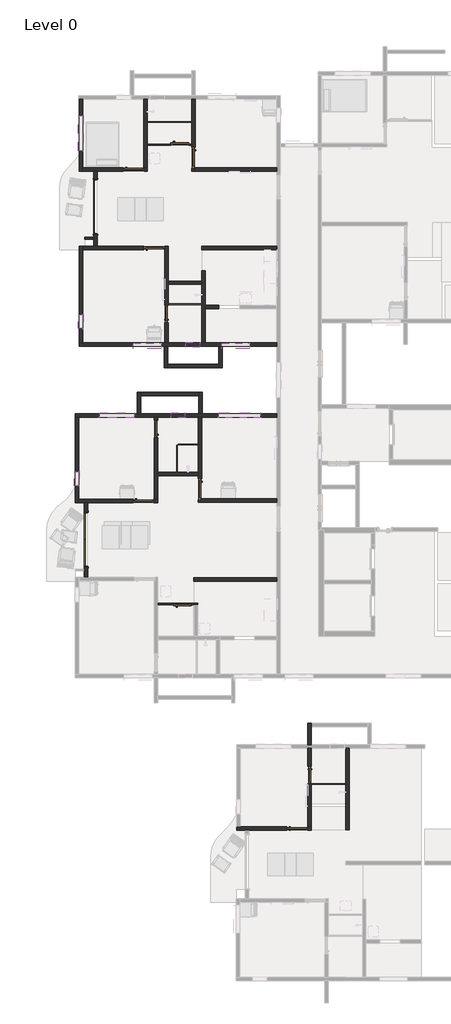
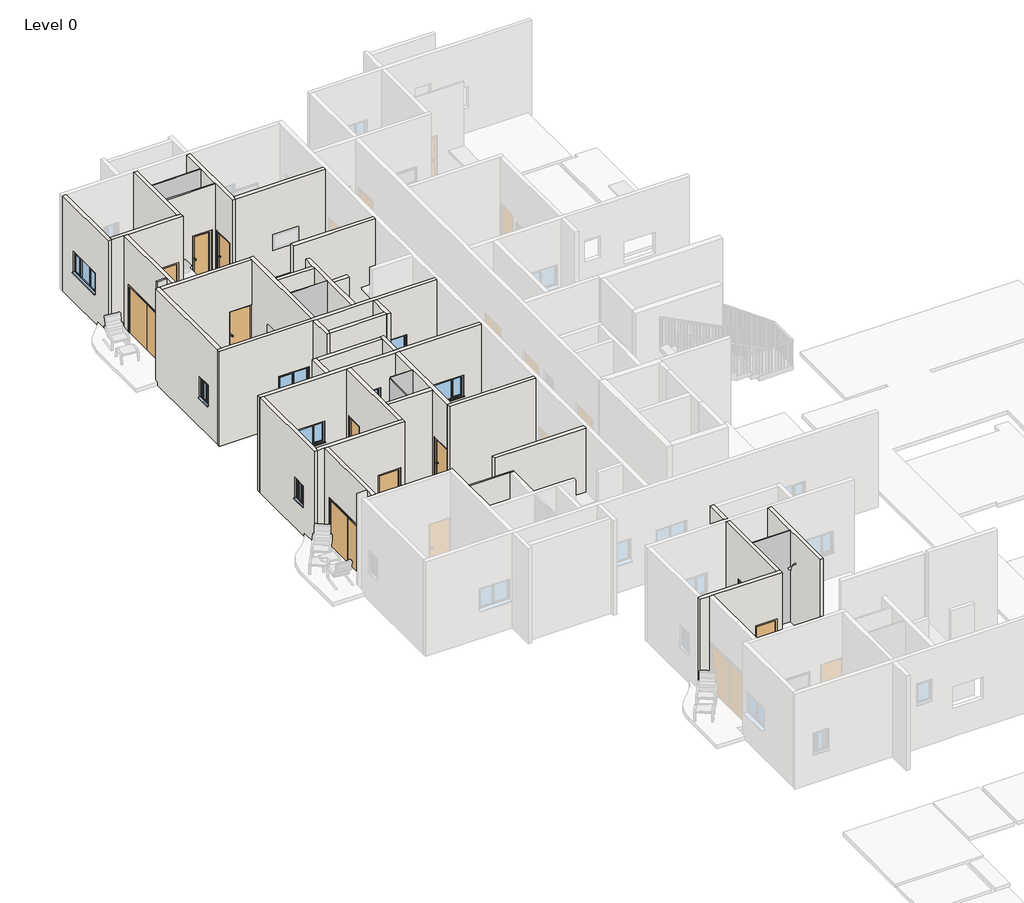
# One storey, part 4 of 14: 35 walls, 14 doors, 9 windows, 5 plates.
"""IFC4 building model written with IfcOpenShell, lengths in millimetres."""

from ifc_helpers import new_model, si_unit, frame, origin, origin_with_axes, place, context, project, spatial, polyline, outline, extrude, faceted_brep, transform, mapped, element, save
from components import doors_concept_intdbl_8_5090a96f, doors_extsgl_flush_d2_fac1298c, doors_extsgl_flush_d2_5e0ff3e2, doors_extsgl_flush_d3_352cde1d, doors_extsgl_flush_d3_ba5ff989, doors_extsgl_flush_d3_fcdd24de, doors_extsgl_flush_d3_225e8ac6, system_panel_glazed_095a6893, system_panel_glazed_930ddd10, system_panel_glazed_c2994357, system_panel_glazed_5123bacf, system_panel_glazed_5cf703a3, windows_concept_plain_dbl_4_d1e2e333, windows_sgl_plain_2_be143095, windows_tpl_variable_casement_2_47b04551, windows_tpl_variable_casement_5_ffad3fa3, windows_tpl_variable_casement_6_d811e495

model = new_model("IFC4")

# Units and contexts
model_context = context("Model", 3, world=origin())
ifc_project = project(units=[si_unit("LENGTHUNIT", "METRE", prefix="MILLI")], contexts=[model_context])

# Site, building, storey
site = spatial("IfcSite", under=ifc_project)
building = spatial("IfcBuilding", under=site)
storey = spatial("IfcBuildingStorey", under=building, Name="Level 0", Elevation=0.0)

# Doors
placement = place(None, origin())
doors_concept_intdbl_8_shape = doors_concept_intdbl_8_5090a96f(model_context)
element("IfcDoor", 1, ObjectType="Doors_Concept_IntDbl : 8'", at=placement, inside=storey, context=model_context, shape_type="MappedRepresentation", body=[
    mapped(doors_concept_intdbl_8_shape, transform((-38935.3458282, 59742.2966928, 0.0), x_axis=(0.0, 1.0, 0.0), y_axis=(-1.0, 0.0, 0.0), z_axis=(0.0, 0.0, 1.0))),
])
element("IfcDoor", 2, ObjectType="Doors_Concept_IntDbl : 8'", at=placement, inside=storey, context=model_context, shape_type="MappedRepresentation", body=[
    mapped(doors_concept_intdbl_8_shape, transform((-39340.8800447, 45143.1998557, 0.0), x_axis=(0.0, 1.0, 0.0), y_axis=(-1.0, 0.0, 0.0), z_axis=(0.0, 0.0, 1.0))),
])
doors_extsgl_flush_d2_shape = doors_extsgl_flush_d2_fac1298c(model_context)
element("IfcDoor", 3, ObjectType="Doors_ExtSgl_Flush : D2", at=placement, inside=storey, context=model_context, shape_type="MappedRepresentation", body=[
    mapped(doors_extsgl_flush_d2_shape, transform((-30080.8505269, 32458.2541094, 0.0), x_axis=(1.0, 0.0, 0.0), y_axis=(0.0, 1.0, 0.0), z_axis=(0.0, 0.0, 1.0))),
])
element("IfcDoor", 4, ObjectType="Doors_ExtSgl_Flush : D2", at=placement, inside=storey, context=model_context, shape_type="MappedRepresentation", body=[
    mapped(doors_extsgl_flush_d2_shape, transform((-36827.1458282, 46838.6498557, 0.0), x_axis=(1.0, 0.0, 0.0), y_axis=(0.0, 1.0, 0.0), z_axis=(0.0, 0.0, 1.0))),
])
element("IfcDoor", 5, ObjectType="Doors_ExtSgl_Flush : D2", at=placement, inside=storey, context=model_context, shape_type="MappedRepresentation", body=[
    mapped(doors_extsgl_flush_d2_shape, transform((-34343.1432055, 47352.8982557, 0.0), x_axis=(0.0, -1.0, 0.0), y_axis=(1.0, 0.0, 0.0), z_axis=(0.0, 0.0, 1.0))),
])
element("IfcDoor", 6, ObjectType="Doors_ExtSgl_Flush : D2", at=placement, inside=storey, context=model_context, shape_type="MappedRepresentation", body=[
    mapped(doors_extsgl_flush_d2_shape, transform((-34631.0273605, 61895.5497514, 0.0), x_axis=(0.0, -1.0, 0.0), y_axis=(1.0, 0.0, 0.0), z_axis=(0.0, 0.0, 1.0))),
])
element("IfcDoor", 7, ObjectType="Doors_ExtSgl_Flush : D2", at=placement, inside=storey, context=model_context, shape_type="MappedRepresentation", body=[
    mapped(doors_extsgl_flush_d2_shape, transform((-37254.3014709, 61386.4998557, 0.0), x_axis=(1.0, 0.0, 0.0), y_axis=(0.0, 1.0, 0.0), z_axis=(0.0, 0.0, 1.0))),
])
doors_extsgl_flush_d2_2_shape = doors_extsgl_flush_d2_5e0ff3e2(model_context)
element("IfcDoor", 8, ObjectType="Doors_ExtSgl_Flush : D2", at=placement, inside=storey, context=model_context, shape_type="MappedRepresentation", body=[
    mapped(doors_extsgl_flush_d2_2_shape, transform((-36348.8695937, 57932.0998557, 0.0), x_axis=(1.0, 0.0, 0.0), y_axis=(0.0, 1.0, 0.0), z_axis=(0.0, 0.0, 1.0))),
])
doors_extsgl_flush_d3_shape = doors_extsgl_flush_d3_352cde1d(model_context)
element("IfcDoor", 9, ObjectType="Doors_ExtSgl_Flush : D3", at=placement, inside=storey, context=model_context, shape_type="MappedRepresentation", body=[
    mapped(doors_extsgl_flush_d3_shape, transform((-29534.6489269, 34807.7541094, 0.0), x_axis=(0.0, -1.0, 0.0), y_axis=(1.0, 0.0, 0.0), z_axis=(0.0, 0.0, 1.0))),
])
doors_extsgl_flush_d3_2_shape = doors_extsgl_flush_d3_ba5ff989(model_context)
element("IfcDoor", 10, ObjectType="Doors_ExtSgl_Flush : D3", at=placement, inside=storey, context=model_context, shape_type="MappedRepresentation", body=[
    mapped(doors_extsgl_flush_d3_2_shape, transform((-36280.9442282, 49994.4982557, 0.0), x_axis=(0.0, 1.0, 0.0), y_axis=(-1.0, 0.0, 0.0), z_axis=(0.0, 0.0, 1.0))),
])
element("IfcDoor", 11, ObjectType="Doors_ExtSgl_Flush : D3", at=placement, inside=storey, context=model_context, shape_type="MappedRepresentation", body=[
    mapped(doors_extsgl_flush_d3_2_shape, transform((-35828.0679937, 55042.7990557, 0.0), x_axis=(0.0, 1.0, 0.0), y_axis=(-1.0, 0.0, 0.0), z_axis=(0.0, 0.0, 1.0))),
])
doors_extsgl_flush_d3_3_shape = doors_extsgl_flush_d3_fcdd24de(model_context)
element("IfcDoor", 12, ObjectType="Doors_ExtSgl_Flush : D3", at=placement, inside=storey, context=model_context, shape_type="MappedRepresentation", body=[
    mapped(doors_extsgl_flush_d3_3_shape, transform((-35113.5855022, 42308.8982471, 0.0), x_axis=(1.0, 0.0, 0.0), y_axis=(0.0, 1.0, 0.0), z_axis=(0.0, 0.0, 1.0))),
])
doors_extsgl_flush_d3_4_shape = doors_extsgl_flush_d3_225e8ac6(model_context)
element("IfcDoor", 13, ObjectType="Doors_ExtSgl_Flush : D3", at=placement, inside=storey, context=model_context, shape_type="MappedRepresentation", body=[
    mapped(doors_extsgl_flush_d3_4_shape, transform((-35228.0289605, 62466.7110557, 0.0), x_axis=(1.0, 0.0, 0.0), y_axis=(0.0, 1.0, 0.0), z_axis=(0.0, 0.0, 1.0))),
])
element("IfcDoor", 14, ObjectType="Doors_ExtSgl_Flush : D3", at=placement, inside=storey, context=model_context, shape_type="MappedRepresentation", body=[
    mapped(doors_extsgl_flush_d3_4_shape, transform((-35253.4289605, 62466.7110557, 0.0), x_axis=(1.0, 0.0, 0.0), y_axis=(0.0, 1.0, 0.0), z_axis=(0.0, 0.0, 1.0))),
])

# Plates
system_panel_glazed_shape = system_panel_glazed_095a6893(model_context)
element("IfcPlate", 15, ObjectType="System Panel : Glazed", at=placement, inside=storey, context=model_context, shape_type="MappedRepresentation", body=[
    mapped(system_panel_glazed_shape, transform((-35312.0437168, 48686.3982557, 0.0), x_axis=(0.0, 1.0, 0.0), y_axis=(-1.0, 0.0, 0.0), z_axis=(0.0, 0.0, 1.0))),
])
system_panel_glazed_2_shape = system_panel_glazed_930ddd10(model_context)
element("IfcPlate", 16, ObjectType="System Panel : Glazed", at=placement, inside=storey, context=model_context, shape_type="MappedRepresentation", body=[
    mapped(system_panel_glazed_2_shape, transform((-34865.6934612, 49283.2982557, 0.0), x_axis=(1.0, 0.0, 0.0), y_axis=(0.0, 1.0, 0.0), z_axis=(0.0, 0.0, 1.0))),
])
system_panel_glazed_3_shape = system_panel_glazed_c2994357(model_context)
element("IfcPlate", 17, ObjectType="System Panel : Glazed", at=placement, inside=storey, context=model_context, shape_type="MappedRepresentation", body=[
    mapped(system_panel_glazed_3_shape, transform((-28705.7468508, 34460.9800488, 0.0), x_axis=(-1.0, 0.0, 0.0), y_axis=(0.0, -1.0, 0.0), z_axis=(0.0, 0.0, 1.0))),
])
system_panel_glazed_4_shape = system_panel_glazed_5123bacf(model_context)
element("IfcPlate", 18, ObjectType="System Panel : Glazed", at=placement, inside=storey, context=model_context, shape_type="MappedRepresentation", body=[
    mapped(system_panel_glazed_4_shape, transform((-35015.2679937, 55500.6170169, 0.0), x_axis=(-1.0, 0.0, 0.0), y_axis=(0.0, -1.0, 0.0), z_axis=(0.0, 0.0, 1.0))),
])
system_panel_glazed_5_shape = system_panel_glazed_5cf703a3(model_context)
element("IfcPlate", 19, ObjectType="System Panel : Glazed", at=placement, inside=storey, context=model_context, shape_type="MappedRepresentation", body=[
    mapped(system_panel_glazed_5_shape, transform((-35682.2636157, 63431.1998557, 0.0), x_axis=(1.0, 0.0, 0.0), y_axis=(0.0, 1.0, 0.0), z_axis=(0.0, 0.0, 1.0))),
])

# Walls
element("IfcWall", 20, ObjectType="W1", at=placement, inside=storey, context=model_context, shape_type="Brep", body=[
    faceted_brep([(-29458.4489269, 32534.4541094, 0.0), (-29610.8489269, 32534.4541094, 0.0), (-29623.6505269, 32534.4541094, 0.0), (-29623.6505269, 32534.4541094, 2110.0), (-30538.0505269, 32534.4541094, 2110.0), (-30538.0505269, 32534.4541094, 0.0), (-32591.6041796, 32534.4541094, 0.0), (-32744.0041796, 32534.4541094, 0.0), (-32744.0041796, 32534.4541094, 4000.0), (-32591.6041796, 32534.4541094, 4000.0), (-29610.8489269, 32534.4541094, 4000.0), (-29458.4489269, 32534.4541094, 4000.0), (-29623.6505269, 32382.0541094, 2110.0), (-29623.6505269, 32382.0541094, 0.0), (-29458.4489269, 32382.0541094, 0.0), (-29458.4489269, 32382.0541094, 4000.0), (-32203.4800447, 32382.0541094, 4000.0), (-32355.8800447, 32382.0541094, 4000.0), (-32744.0041796, 32382.0541094, 4000.0), (-32744.0041796, 32382.0541094, 0.0), (-32355.8800447, 32382.0541094, 0.0), (-32203.4800447, 32382.0541094, 0.0), (-30538.0505269, 32382.0541094, 0.0), (-30538.0505269, 32382.0541094, 2110.0)], [[[0, 1, 2, 3, 4, 5, 6, 7, 8, 9, 10, 11]], [[12, 13, 14, 15, 16, 17, 18, 19, 20, 21, 22, 23]], [[14, 13, 2, 1, 0]], [[22, 21, 20, 19, 7, 6, 5]], [[11, 10, 9, 8, 18, 17, 16, 15]], [[8, 7, 19, 18]], [[0, 11, 15, 14]], [[5, 4, 23, 22]], [[3, 2, 13, 12]], [[4, 3, 12, 23]]]),
])
element("IfcWall", 21, ObjectType="W1", at=placement, inside=storey, context=model_context, shape_type="Brep", body=[
    faceted_brep([(-29458.4489269, 32534.4541094, 4000.0), (-29458.4489269, 32534.4541094, 0.0), (-29458.4489269, 34426.7541094, 0.0), (-29458.4489269, 34426.7541094, 2110.0), (-29458.4489269, 35188.7541094, 2110.0), (-29458.4489269, 35188.7541094, 0.0), (-29458.4489269, 35984.9800488, 0.0), (-29458.4489269, 35984.9800488, 4000.0), (-29610.8489269, 32534.4541094, 0.0), (-29610.8489269, 32534.4541094, 4000.0), (-29610.8489269, 35984.9800488, 4000.0), (-29610.8489269, 35984.9800488, 0.0), (-29610.8489269, 35188.7541094, 0.0), (-29610.8489269, 35188.7541094, 2110.0), (-29610.8489269, 34426.7541094, 2110.0), (-29610.8489269, 34426.7541094, 0.0)], [[[0, 1, 2, 3, 4, 5, 6, 7]], [[8, 9, 10, 11, 12, 13, 14, 15]], [[1, 8, 15, 2]], [[5, 12, 11, 6]], [[9, 0, 7, 10]], [[1, 0, 9, 8]], [[7, 6, 11, 10]], [[5, 4, 13, 12]], [[3, 2, 15, 14]], [[4, 3, 14, 13]]]),
    faceted_brep([(-29458.4489269, 37081.0541094, 0.0), (-29458.4489269, 37081.0541094, 4000.0), (-29458.4489269, 36928.6541094, 4000.0), (-29458.4489269, 36137.3800488, 4000.0), (-29458.4489269, 36137.3800488, 0.0), (-29458.4489269, 36928.6541094, 0.0), (-29610.8489269, 37081.0541094, 4000.0), (-29610.8489269, 37081.0541094, 0.0), (-29610.8489269, 36137.3800488, 0.0), (-29610.8489269, 36137.3800488, 4000.0)], [[[0, 1, 2, 3, 4, 5]], [[6, 7, 8, 9]], [[7, 0, 5, 4, 8]], [[1, 6, 9, 3, 2]], [[4, 3, 9, 8]], [[1, 0, 7, 6]]]),
])
element("IfcWall", 22, ObjectType="W1", at=placement, inside=storey, context=model_context, shape_type="SweptSolid", body=[
    extrude(outline(polyline([(-27800.6447747, 35984.9800488), (-27800.6447747, 32399.4161504), (-27953.0447747, 32399.4161504), (-27953.0447747, 35984.9800488), (-27800.6447747, 35984.9800488)])), origin_with_axes(), (0.0, 0.0, 1.0), 4000.0),
])
element("IfcWall", 23, ObjectType="W1", at=placement, inside=storey, context=model_context, shape_type="Brep", body=[
    faceted_brep([(-39264.6800447, 46762.4498557, 4000.0), (-39264.6800447, 43479.4998557, 4000.0), (-39264.6800447, 43479.4998557, 0.0), (-39264.6800447, 43923.9998557, 0.0), (-39264.6800447, 43923.9998557, 2110.0), (-39264.6800447, 46362.3998557, 2110.0), (-39264.6800447, 46362.3998557, 0.0), (-39264.6800447, 46762.4498557, 0.0), (-39417.0800447, 43479.4998557, 4000.0), (-39417.0800447, 43778.0006557, 4000.0), (-39417.0800447, 43847.7998557, 4000.0), (-39417.0800447, 46762.4498557, 4000.0), (-39417.0800447, 46762.4498557, 0.0), (-39417.0800447, 46362.3998557, 0.0), (-39417.0800447, 46362.3998557, 2110.0), (-39417.0800447, 43923.9998557, 2110.0), (-39417.0800447, 43923.9998557, 0.0), (-39417.0800447, 43847.7998557, 0.0), (-39417.0800447, 43778.0006557, 0.0), (-39417.0800447, 43479.4998557, 0.0)], [[[0, 1, 2, 3, 4, 5, 6, 7]], [[8, 9, 10, 11, 12, 13, 14, 15, 16, 17, 18, 19]], [[2, 19, 18, 17, 16, 3]], [[12, 7, 6, 13]], [[1, 0, 11, 10, 9, 8]], [[2, 1, 8, 19]], [[0, 7, 12, 11]], [[5, 14, 13, 6]], [[14, 5, 4, 15]], [[15, 4, 3, 16]]]),
])
element("IfcWall", 24, ObjectType="W1", at=placement, inside=storey, context=model_context, shape_type="SweptSolid", body=[
    extrude(outline(polyline([(-34617.3458282, 43460.4498557), (-30972.3442282, 43460.4498557), (-30972.3442282, 43308.0498557), (-34617.3458282, 43308.0498557), (-34617.3458282, 43460.4498557)])), origin_with_axes(), (0.0, 0.0, 1.0), 4000.0),
])
element("IfcWall", 25, ObjectType="W1", at=placement, inside=storey, context=model_context, shape_type="Brep", body=[
    faceted_brep([(-30972.3442282, 50667.6998557, 0.0), (-34247.8932055, 50667.6998557, 0.0), (-34400.2932055, 50667.6998557, 0.0), (-36954.1458282, 50667.6998557, 0.0), (-37106.5458282, 50667.6998557, 0.0), (-39824.3458282, 50667.6998557, 0.0), (-39824.3458282, 50667.6998557, 4000.0), (-37106.5458282, 50667.6998557, 4000.0), (-36954.1458282, 50667.6998557, 4000.0), (-34400.2932055, 50667.6998557, 4000.0), (-34247.8932055, 50667.6998557, 4000.0), (-30972.3442282, 50667.6998557, 4000.0), (-38757.5458282, 50667.6998557, 2110.0), (-38757.5458282, 50667.6998557, 1200.0), (-37233.5458282, 50667.6998557, 1200.0), (-37233.5458282, 50667.6998557, 2110.0), (-33524.5187168, 50667.6998557, 2110.0), (-33524.5187168, 50667.6998557, 1200.0), (-31695.7187168, 50667.6998557, 1200.0), (-31695.7187168, 50667.6998557, 2110.0), (-35616.8437168, 50667.6998557, 2738.9328), (-35616.8437168, 50667.6998557, 1828.9328), (-35007.2437168, 50667.6998557, 1828.9328), (-35007.2437168, 50667.6998557, 2738.9328), (-30972.3442282, 50515.2998557, 0.0), (-30972.3442282, 50515.2998557, 4000.0), (-34266.9432055, 50515.2998557, 4000.0), (-34419.3432055, 50515.2998557, 4000.0), (-36204.7442282, 50515.2998557, 4000.0), (-36357.1442282, 50515.2998557, 4000.0), (-39671.9458282, 50515.2998557, 4000.0), (-39824.3458282, 50515.2998557, 4000.0), (-39824.3458282, 50515.2998557, 0.0), (-39671.9458282, 50515.2998557, 0.0), (-36357.1442282, 50515.2998557, 0.0), (-36204.7442282, 50515.2998557, 0.0), (-34419.3432055, 50515.2998557, 0.0), (-34266.9432055, 50515.2998557, 0.0), (-38757.5458282, 50515.2998557, 2110.0), (-37233.5458282, 50515.2998557, 2110.0), (-37233.5458282, 50515.2998557, 1200.0), (-38757.5458282, 50515.2998557, 1200.0), (-33524.5187168, 50515.2998557, 2110.0), (-31695.7187168, 50515.2998557, 2110.0), (-31695.7187168, 50515.2998557, 1200.0), (-33524.5187168, 50515.2998557, 1200.0), (-35616.8437168, 50515.2998557, 2738.9328), (-35007.2437168, 50515.2998557, 2738.9328), (-35007.2437168, 50515.2998557, 1828.9328), (-35616.8437168, 50515.2998557, 1828.9328)], [[[0, 1, 2, 3, 4, 5, 6, 7, 8, 9, 10, 11], [12, 13, 14, 15], [16, 17, 18, 19], [20, 21, 22, 23]], [[24, 25, 26, 27, 28, 29, 30, 31, 32, 33, 34, 35, 36, 37], [38, 39, 40, 41], [42, 43, 44, 45], [46, 47, 48, 49]], [[5, 4, 3, 2, 1, 0, 24, 37, 36, 35, 34, 33, 32]], [[11, 10, 9, 8, 7, 6, 31, 30, 29, 28, 27, 26, 25]], [[0, 11, 25, 24]], [[6, 5, 32, 31]], [[13, 12, 38, 41]], [[14, 13, 41, 40]], [[15, 14, 40, 39]], [[12, 15, 39, 38]], [[17, 16, 42, 45]], [[18, 17, 45, 44]], [[19, 18, 44, 43]], [[16, 19, 43, 42]], [[21, 20, 46, 49]], [[22, 21, 49, 48]], [[23, 22, 48, 47]], [[20, 23, 47, 46]]]),
])
element("IfcWall", 26, ObjectType="W1", at=placement, inside=storey, context=model_context, shape_type="Brep", body=[
    faceted_brep([(-39824.3458282, 50515.2998557, 0.0), (-39824.3458282, 46762.4498557, 0.0), (-39824.3458282, 46762.4498557, 4000.0), (-39824.3458282, 50515.2998557, 4000.0), (-39824.3458282, 47499.0498557, 2110.0), (-39824.3458282, 47499.0498557, 1200.0), (-39824.3458282, 48108.6498557, 1200.0), (-39824.3458282, 48108.6498557, 2110.0), (-39671.9458282, 50515.2998557, 0.0), (-39671.9458282, 50515.2998557, 4000.0), (-39671.9458282, 46914.8498557, 4000.0), (-39671.9458282, 46762.4498557, 4000.0), (-39671.9458282, 46762.4498557, 0.0), (-39671.9458282, 46914.8498557, 0.0), (-39671.9458282, 47499.0498557, 2110.0), (-39671.9458282, 48108.6498557, 2110.0), (-39671.9458282, 48108.6498557, 1200.0), (-39671.9458282, 47499.0498557, 1200.0)], [[[0, 1, 2, 3], [4, 5, 6, 7]], [[8, 9, 10, 11, 12, 13], [14, 15, 16, 17]], [[1, 0, 8, 13, 12]], [[3, 2, 11, 10, 9]], [[0, 3, 9, 8]], [[2, 1, 12, 11]], [[5, 4, 14, 17]], [[6, 5, 17, 16]], [[7, 6, 16, 15]], [[4, 7, 15, 14]]]),
])
element("IfcWall", 27, ObjectType="W1", at=placement, inside=storey, context=model_context, shape_type="Brep", body=[
    faceted_brep([(-36369.9458282, 46762.4498557, 2110.0), (-36369.9458282, 46762.4498557, 0.0), (-36204.7442282, 46762.4498557, 0.0), (-36204.7442282, 46762.4498557, 4000.0), (-39264.6800447, 46762.4498557, 4000.0), (-39417.0800447, 46762.4498557, 4000.0), (-39671.9458282, 46762.4498557, 4000.0), (-39671.9458282, 46762.4498557, 0.0), (-39417.0800447, 46762.4498557, 0.0), (-39264.6800447, 46762.4498557, 0.0), (-37284.3458282, 46762.4498557, 0.0), (-37284.3458282, 46762.4498557, 2110.0), (-36204.7442282, 46914.8498557, 0.0), (-36357.1442282, 46914.8498557, 0.0), (-36369.9458282, 46914.8498557, 0.0), (-36369.9458282, 46914.8498557, 2110.0), (-37284.3458282, 46914.8498557, 2110.0), (-37284.3458282, 46914.8498557, 0.0), (-39671.9458282, 46914.8498557, 0.0), (-39671.9458282, 46914.8498557, 4000.0), (-36357.1442282, 46914.8498557, 4000.0), (-36204.7442282, 46914.8498557, 4000.0)], [[[0, 1, 2, 3, 4, 5, 6, 7, 8, 9, 10, 11]], [[12, 13, 14, 15, 16, 17, 18, 19, 20, 21]], [[2, 1, 14, 13, 12]], [[10, 9, 8, 7, 18, 17]], [[6, 5, 4, 3, 21, 20, 19]], [[7, 6, 19, 18]], [[3, 2, 12, 21]], [[17, 16, 11, 10]], [[15, 14, 1, 0]], [[16, 15, 0, 11]]]),
])
element("IfcWall", 28, ObjectType="W1", at=placement, inside=storey, context=model_context, shape_type="Brep", body=[
    faceted_brep([(-36204.7442282, 50375.4982557, 2110.0), (-36204.7442282, 50375.4982557, 0.0), (-36204.7442282, 50515.2998557, 0.0), (-36204.7442282, 50515.2998557, 4000.0), (-36204.7442282, 48089.4982557, 4000.0), (-36204.7442282, 47937.0982557, 4000.0), (-36204.7442282, 46914.8498557, 4000.0), (-36204.7442282, 46914.8498557, 0.0), (-36204.7442282, 47937.0982557, 0.0), (-36204.7442282, 48089.4982557, 0.0), (-36204.7442282, 49613.4982557, 0.0), (-36204.7442282, 49613.4982557, 2110.0), (-36357.1442282, 50515.2998557, 0.0), (-36357.1442282, 50375.4982557, 0.0), (-36357.1442282, 50375.4982557, 2110.0), (-36357.1442282, 49613.4982557, 2110.0), (-36357.1442282, 49613.4982557, 0.0), (-36357.1442282, 46914.8498557, 0.0), (-36357.1442282, 46914.8498557, 4000.0), (-36357.1442282, 50515.2998557, 4000.0)], [[[0, 1, 2, 3, 4, 5, 6, 7, 8, 9, 10, 11]], [[12, 13, 14, 15, 16, 17, 18, 19]], [[2, 1, 13, 12]], [[10, 9, 8, 7, 17, 16]], [[6, 5, 4, 3, 19, 18]], [[7, 6, 18, 17]], [[3, 2, 12, 19]], [[16, 15, 11, 10]], [[14, 13, 1, 0]], [[15, 14, 0, 11]]]),
])
element("IfcWall", 29, ObjectType="W1", at=placement, inside=storey, context=model_context, shape_type="Brep", body=[
    faceted_brep([(-34419.3432055, 46921.0982557, 4000.0), (-34419.3432055, 47937.0982557, 4000.0), (-34419.3432055, 48089.4982557, 4000.0), (-34419.3432055, 50515.2998557, 4000.0), (-34419.3432055, 50515.2998557, 0.0), (-34419.3432055, 48089.4982557, 0.0), (-34419.3432055, 47937.0982557, 0.0), (-34419.3432055, 47810.0982557, 0.0), (-34419.3432055, 47810.0982557, 2110.0), (-34419.3432055, 46921.0982557, 2110.0), (-34266.9432055, 50515.2998557, 4000.0), (-34266.9432055, 46921.0982557, 4000.0), (-34266.9432055, 46921.0982557, 2110.0), (-34266.9432055, 47810.0982557, 2110.0), (-34266.9432055, 47810.0982557, 0.0), (-34266.9432055, 50515.2998557, 0.0)], [[[0, 1, 2, 3, 4, 5, 6, 7, 8, 9]], [[10, 11, 12, 13, 14, 15]], [[4, 15, 14, 7, 6, 5]], [[3, 2, 1, 0, 11, 10]], [[4, 3, 10, 15]], [[11, 0, 9, 12]], [[13, 8, 7, 14]], [[8, 13, 12, 9]]]),
])
element("IfcWall", 30, ObjectType="W1", at=placement, inside=storey, context=model_context, shape_type="SweptSolid", body=[
    extrude(outline(polyline([(-36204.7442282, 48089.4982557), (-34419.3432055, 48089.4982557), (-34419.3432055, 47937.0982557), (-36204.7442282, 47937.0982557), (-36204.7442282, 48089.4982557)])), origin_with_axes(), (0.0, 0.0, 1.0), 4000.0),
])
element("IfcWall", 31, ObjectType="W1", at=placement, inside=storey, context=model_context, shape_type="Brep", body=[
    faceted_brep([(-34419.3432055, 46921.0982557, 4000.0), (-34266.9432055, 46921.0982557, 4000.0), (-30972.3442282, 46921.0982557, 4000.0), (-30972.3442282, 46921.0982557, 0.0), (-34266.9432055, 46921.0982557, 0.0), (-34266.9432055, 46921.0982557, 2110.0), (-34419.3432055, 46921.0982557, 2110.0), (-34419.3432055, 46768.6982557, 0.0), (-30972.3442282, 46768.6982557, 0.0), (-30972.3442282, 46768.6982557, 4000.0), (-34419.3432055, 46768.6982557, 4000.0), (-34419.3432055, 46895.6982557, 0.0), (-34266.9432055, 46895.6982557, 0.0), (-34419.3432055, 46895.6982557, 2110.0), (-34266.9432055, 46895.6982557, 2110.0)], [[[0, 1, 2, 3, 4, 5, 6]], [[7, 8, 9, 10]], [[8, 7, 11, 12, 4, 3]], [[2, 1, 0, 10, 9]], [[3, 2, 9, 8]], [[7, 10, 0, 6, 13, 11]], [[12, 14, 5, 4]], [[14, 12, 11, 13]], [[14, 13, 6, 5]]]),
])
element("IfcWall", 32, ObjectType="W1", at=placement, inside=storey, context=model_context, shape_type="Brep", body=[
    faceted_brep([(-36954.1458282, 50667.6998557, 0.0), (-36954.1458282, 51448.6990557, 0.0), (-36954.1458282, 51601.0990557, 0.0), (-36954.1458282, 51601.0990557, 4000.0), (-36954.1458282, 51448.6990557, 4000.0), (-36954.1458282, 50667.6998557, 4000.0), (-37106.5458282, 50667.6998557, 0.0), (-37106.5458282, 50667.6998557, 4000.0), (-37106.5458282, 51601.0990557, 4000.0), (-37106.5458282, 51601.0990557, 0.0)], [[[0, 1, 2, 3, 4, 5]], [[6, 7, 8, 9]], [[2, 1, 0, 6, 9]], [[5, 4, 3, 8, 7]], [[0, 5, 7, 6]], [[3, 2, 9, 8]]]),
])
element("IfcWall", 33, ObjectType="W1", at=placement, inside=storey, context=model_context, shape_type="Brep", body=[
    faceted_brep([(-34247.8932055, 50667.6998557, 0.0), (-34247.8932055, 51607.4998557, 0.0), (-34247.8932055, 51607.4998557, 4000.0), (-34247.8932055, 50667.6998557, 4000.0), (-34400.2932055, 50667.6998557, 0.0), (-34400.2932055, 50667.6998557, 4000.0), (-34400.2932055, 51448.6990557, 4000.0), (-34400.2932055, 51601.0990557, 4000.0), (-34400.2932055, 51607.4998557, 4000.0), (-34400.2932055, 51607.4998557, 0.0), (-34400.2932055, 51601.0990557, 0.0), (-34400.2932055, 51448.6990557, 0.0)], [[[0, 1, 2, 3]], [[4, 5, 6, 7, 8, 9, 10, 11]], [[1, 0, 4, 11, 10, 9]], [[2, 1, 9, 8]], [[3, 2, 8, 7, 6, 5]], [[0, 3, 5, 4]]]),
])
element("IfcWall", 34, ObjectType="W1", at=placement, inside=storey, context=model_context, shape_type="Brep", body=[
    faceted_brep([(-30972.3442282, 53766.4998557, 0.0), (-34126.2679937, 53766.4998557, 0.0), (-34278.6679937, 53766.4998557, 0.0), (-35751.8679937, 53766.4998557, 0.0), (-35904.2679937, 53766.4998557, 0.0), (-39494.1458282, 53766.4998557, 0.0), (-39646.5458282, 53766.4998557, 0.0), (-39646.5458282, 53766.4998557, 4000.0), (-39494.1458282, 53766.4998557, 4000.0), (-35904.2679937, 53766.4998557, 4000.0), (-35751.8679937, 53766.4998557, 4000.0), (-34278.6679937, 53766.4998557, 4000.0), (-34126.2679937, 53766.4998557, 4000.0), (-30972.3442282, 53766.4998557, 4000.0), (-36056.6679937, 53766.4998557, 2110.0), (-37275.8679937, 53766.4998557, 2110.0), (-37275.8679937, 53766.4998557, 1200.0), (-36056.6679937, 53766.4998557, 1200.0), (-32170.4679937, 53766.4998557, 2110.0), (-33389.6679937, 53766.4998557, 2110.0), (-33389.6679937, 53766.4998557, 1200.0), (-32170.4679937, 53766.4998557, 1200.0), (-34354.8679937, 53766.4998557, 2738.9328), (-34964.4679937, 53766.4998557, 2738.9328), (-34964.4679937, 53766.4998557, 1828.9328), (-34354.8679937, 53766.4998557, 1828.9328), (-30972.3442282, 53614.0998557, 0.0), (-30972.3442282, 53614.0998557, 4000.0), (-33364.2679937, 53614.0998557, 4000.0), (-33516.6679937, 53614.0998557, 4000.0), (-35764.5679937, 53614.0998557, 4000.0), (-35916.9679937, 53614.0998557, 4000.0), (-39646.5458282, 53614.0998557, 4000.0), (-39646.5458282, 53614.0998557, 0.0), (-35916.9679937, 53614.0998557, 0.0), (-35764.5679937, 53614.0998557, 0.0), (-33516.6679937, 53614.0998557, 0.0), (-33364.2679937, 53614.0998557, 0.0), (-36056.6679937, 53614.0998557, 2110.0), (-36056.6679937, 53614.0998557, 1200.0), (-37275.8679937, 53614.0998557, 1200.0), (-37275.8679937, 53614.0998557, 2110.0), (-32170.4679937, 53614.0998557, 2110.0), (-32170.4679937, 53614.0998557, 1200.0), (-33389.6679937, 53614.0998557, 1200.0), (-33389.6679937, 53614.0998557, 2110.0), (-34354.8679937, 53614.0998557, 2738.9328), (-34354.8679937, 53614.0998557, 1828.9328), (-34964.4679937, 53614.0998557, 1828.9328), (-34964.4679937, 53614.0998557, 2738.9328)], [[[0, 1, 2, 3, 4, 5, 6, 7, 8, 9, 10, 11, 12, 13], [14, 15, 16, 17], [18, 19, 20, 21], [22, 23, 24, 25]], [[26, 27, 28, 29, 30, 31, 32, 33, 34, 35, 36, 37], [38, 39, 40, 41], [42, 43, 44, 45], [46, 47, 48, 49]], [[6, 5, 4, 3, 2, 1, 0, 26, 37, 36, 35, 34, 33]], [[13, 12, 11, 10, 9, 8, 7, 32, 31, 30, 29, 28, 27]], [[0, 13, 27, 26]], [[7, 6, 33, 32]], [[39, 38, 14, 17]], [[40, 39, 17, 16]], [[41, 40, 16, 15]], [[38, 41, 15, 14]], [[43, 42, 18, 21]], [[44, 43, 21, 20]], [[45, 44, 20, 19]], [[42, 45, 19, 18]], [[47, 46, 22, 25]], [[48, 47, 25, 24]], [[49, 48, 24, 23]], [[46, 49, 23, 22]]]),
])
element("IfcWall", 35, ObjectType="W1", at=placement, inside=storey, context=model_context, shape_type="Brep", body=[
    faceted_brep([(-39494.1458282, 53766.4998557, 0.0), (-39494.1458282, 57855.8998557, 0.0), (-39494.1458282, 58008.2998557, 0.0), (-39494.1458282, 58008.2998557, 4000.0), (-39494.1458282, 57855.8998557, 4000.0), (-39494.1458282, 53766.4998557, 4000.0), (-39494.1458282, 54401.4998557, 2110.0), (-39494.1458282, 55011.0998557, 2110.0), (-39494.1458282, 55011.0998557, 1200.0), (-39494.1458282, 54401.4998557, 1200.0), (-39646.5458282, 53766.4998557, 0.0), (-39646.5458282, 53766.4998557, 4000.0), (-39646.5458282, 58008.2998557, 4000.0), (-39646.5458282, 58008.2998557, 0.0), (-39646.5458282, 54401.4998557, 2110.0), (-39646.5458282, 54401.4998557, 1200.0), (-39646.5458282, 55011.0998557, 1200.0), (-39646.5458282, 55011.0998557, 2110.0)], [[[0, 1, 2, 3, 4, 5], [6, 7, 8, 9]], [[10, 11, 12, 13], [14, 15, 16, 17]], [[2, 1, 0, 10, 13]], [[5, 4, 3, 12, 11]], [[0, 5, 11, 10]], [[3, 2, 13, 12]], [[15, 14, 6, 9]], [[16, 15, 9, 8]], [[17, 16, 8, 7]], [[14, 17, 7, 6]]]),
])
element("IfcWall", 36, ObjectType="W1", at=placement, inside=storey, context=model_context, shape_type="Brep", body=[
    faceted_brep([(-35751.8679937, 55423.7990557, 2110.0), (-35751.8679937, 55423.7990557, 0.0), (-35751.8679937, 56331.8998557, 0.0), (-35751.8679937, 56484.2998557, 0.0), (-35751.8679937, 58008.2998557, 0.0), (-35751.8679937, 58008.2998557, 4000.0), (-35751.8679937, 56484.2998557, 4000.0), (-35751.8679937, 56331.8998557, 4000.0), (-35751.8679937, 53766.4998557, 4000.0), (-35751.8679937, 53766.4998557, 0.0), (-35751.8679937, 54661.7990557, 0.0), (-35751.8679937, 54661.7990557, 2110.0), (-35904.2679937, 57855.8998557, 0.0), (-35904.2679937, 55423.7990557, 0.0), (-35904.2679937, 55423.7990557, 2110.0), (-35904.2679937, 54661.7990557, 2110.0), (-35904.2679937, 54661.7990557, 0.0), (-35904.2679937, 53766.4998557, 0.0), (-35904.2679937, 53766.4998557, 4000.0), (-35904.2679937, 57855.8998557, 4000.0), (-35904.2679937, 58008.2998557, 4000.0), (-35904.2679937, 58008.2998557, 2110.0), (-35904.2679937, 57855.8998557, 2110.0), (-35891.6695937, 57855.8998557, 0.0), (-35891.6695937, 58008.2998557, 0.0), (-35891.6695937, 58008.2998557, 2110.0), (-35891.6695937, 57855.8998557, 2110.0)], [[[0, 1, 2, 3, 4, 5, 6, 7, 8, 9, 10, 11]], [[12, 13, 14, 15, 16, 17, 18, 19, 20, 21, 22]], [[10, 9, 17, 16]], [[4, 3, 2, 1, 13, 12, 23, 24]], [[8, 7, 6, 5, 20, 19, 18]], [[9, 8, 18, 17]], [[5, 4, 24, 25, 21, 20]], [[26, 23, 12, 22]], [[23, 26, 25, 24]], [[25, 26, 22, 21]], [[16, 15, 11, 10]], [[14, 13, 1, 0]], [[15, 14, 0, 11]]]),
])
element("IfcWall", 37, ObjectType="W1", at=placement, inside=storey, context=model_context, shape_type="Brep", body=[
    faceted_brep([(-35904.2679937, 57855.8998557, 4000.0), (-39494.1458282, 57855.8998557, 4000.0), (-39494.1458282, 57855.8998557, 0.0), (-36806.0695937, 57855.8998557, 0.0), (-36806.0695937, 57855.8998557, 2110.0), (-35904.2679937, 57855.8998557, 2110.0), (-39494.1458282, 58008.2998557, 4000.0), (-39011.5458282, 58008.2998557, 4000.0), (-38859.1458282, 58008.2998557, 4000.0), (-35904.2679937, 58008.2998557, 4000.0), (-35904.2679937, 58008.2998557, 2110.0), (-36806.0695937, 58008.2998557, 2110.0), (-36806.0695937, 58008.2998557, 0.0), (-38859.1458282, 58008.2998557, 0.0), (-39011.5458282, 58008.2998557, 0.0), (-39494.1458282, 58008.2998557, 0.0)], [[[0, 1, 2, 3, 4, 5]], [[6, 7, 8, 9, 10, 11, 12, 13, 14, 15]], [[2, 15, 14, 13, 12, 3]], [[1, 0, 9, 8, 7, 6]], [[2, 1, 6, 15]], [[9, 0, 5, 10]], [[11, 4, 3, 12]], [[4, 11, 10, 5]]]),
])
element("IfcWall", 38, ObjectType="W1", at=placement, inside=storey, context=model_context, shape_type="Brep", body=[
    faceted_brep([(-34126.2679937, 53766.4998557, 0.0), (-34126.2679937, 55272.0170169, 0.0), (-34126.2679937, 55424.4170169, 0.0), (-34126.2679937, 56941.4998557, 0.0), (-34126.2679937, 56941.4998557, 4000.0), (-34126.2679937, 55424.4170169, 4000.0), (-34126.2679937, 55272.0170169, 4000.0), (-34126.2679937, 53766.4998557, 4000.0), (-34278.6679937, 53766.4998557, 0.0), (-34278.6679937, 53766.4998557, 4000.0), (-34278.6679937, 56331.8998557, 4000.0), (-34278.6679937, 56484.2998557, 4000.0), (-34278.6679937, 56941.4998557, 4000.0), (-34278.6679937, 56941.4998557, 0.0), (-34278.6679937, 56484.2998557, 0.0), (-34278.6679937, 56331.8998557, 0.0)], [[[0, 1, 2, 3, 4, 5, 6, 7]], [[8, 9, 10, 11, 12, 13, 14, 15]], [[3, 2, 1, 0, 8, 15, 14, 13]], [[4, 3, 13, 12]], [[7, 6, 5, 4, 12, 11, 10, 9]], [[0, 7, 9, 8]]]),
])
element("IfcWall", 39, ObjectType="W1", at=placement, inside=storey, context=model_context, shape_type="SweptSolid", body=[
    extrude(outline(polyline([(-34278.6679937, 56331.8998557), (-35751.8679937, 56331.8998557), (-35751.8679937, 56484.2998557), (-34278.6679937, 56484.2998557), (-34278.6679937, 56331.8998557)])), origin_with_axes(), (0.0, 0.0, 1.0), 4000.0),
])
element("IfcWall", 40, ObjectType="W1", at=placement, inside=storey, context=model_context, shape_type="SweptSolid", body=[
    extrude(outline(polyline([(-34261.7458282, 58008.2998557), (-30972.3442282, 58008.2998557), (-30972.3442282, 57855.8998557), (-34261.7458282, 57855.8998557), (-34261.7458282, 58008.2998557)])), origin_with_axes(), (0.0, 0.0, 1.0), 4000.0),
])
element("IfcWall", 41, ObjectType="W1", at=placement, inside=storey, context=model_context, shape_type="Brep", body=[
    faceted_brep([(-38859.1458282, 61310.2998557, 4000.0), (-38859.1458282, 58008.2998557, 4000.0), (-38859.1458282, 58008.2998557, 0.0), (-38859.1458282, 58523.0966928, 0.0), (-38859.1458282, 58523.0966928, 2110.0), (-38859.1458282, 60961.4966928, 2110.0), (-38859.1458282, 60961.4966928, 0.0), (-38859.1458282, 61310.2998557, 0.0), (-39011.5458282, 58008.2998557, 4000.0), (-39011.5458282, 58326.2974928, 4000.0), (-39011.5458282, 58396.0966928, 4000.0), (-39011.5458282, 61310.2998557, 4000.0), (-39011.5458282, 61310.2998557, 0.0), (-39011.5458282, 60961.4966928, 0.0), (-39011.5458282, 60961.4966928, 2110.0), (-39011.5458282, 58523.0966928, 2110.0), (-39011.5458282, 58523.0966928, 0.0), (-39011.5458282, 58396.0966928, 0.0), (-39011.5458282, 58326.2974928, 0.0), (-39011.5458282, 58008.2998557, 0.0)], [[[0, 1, 2, 3, 4, 5, 6, 7]], [[8, 9, 10, 11, 12, 13, 14, 15, 16, 17, 18, 19]], [[2, 19, 18, 17, 16, 3]], [[12, 7, 6, 13]], [[1, 0, 11, 10, 9, 8]], [[2, 1, 8, 19]], [[0, 7, 12, 11]], [[5, 14, 13, 6]], [[14, 5, 4, 15]], [[15, 4, 3, 16]]]),
])
element("IfcWall", 42, ObjectType="W1", at=placement, inside=storey, context=model_context, shape_type="Brep", body=[
    faceted_brep([(-39646.5458282, 64459.8998557, 0.0), (-39646.5458282, 61310.2998557, 0.0), (-39646.5458282, 61310.2998557, 4000.0), (-39646.5458282, 64459.8998557, 4000.0), (-39646.5458282, 62199.2998557, 2110.0), (-39646.5458282, 62199.2998557, 1200.0), (-39646.5458282, 63723.2998557, 1200.0), (-39646.5458282, 63723.2998557, 2110.0), (-39494.1458282, 64459.8998557, 0.0), (-39494.1458282, 64459.8998557, 4000.0), (-39494.1458282, 61462.6998557, 4000.0), (-39494.1458282, 61310.2998557, 4000.0), (-39494.1458282, 61310.2998557, 0.0), (-39494.1458282, 61462.6998557, 0.0), (-39494.1458282, 62199.2998557, 2110.0), (-39494.1458282, 63723.2998557, 2110.0), (-39494.1458282, 63723.2998557, 1200.0), (-39494.1458282, 62199.2998557, 1200.0)], [[[0, 1, 2, 3], [4, 5, 6, 7]], [[8, 9, 10, 11, 12, 13], [14, 15, 16, 17]], [[1, 0, 8, 13, 12]], [[3, 2, 11, 10, 9]], [[0, 3, 9, 8]], [[2, 1, 12, 11]], [[5, 4, 14, 17]], [[6, 5, 17, 16]], [[7, 6, 16, 15]], [[4, 7, 15, 14]]]),
])
element("IfcWall", 43, ObjectType="W1", at=placement, inside=storey, context=model_context, shape_type="Brep", body=[
    faceted_brep([(-36797.1014709, 61310.2998557, 2110.0), (-36797.1014709, 61310.2998557, 0.0), (-36657.2998709, 61310.2998557, 0.0), (-36657.2998709, 61310.2998557, 4000.0), (-38859.1458282, 61310.2998557, 4000.0), (-39011.5458282, 61310.2998557, 4000.0), (-39494.1458282, 61310.2998557, 4000.0), (-39494.1458282, 61310.2998557, 0.0), (-39011.5458282, 61310.2998557, 0.0), (-38859.1458282, 61310.2998557, 0.0), (-37711.5014709, 61310.2998557, 0.0), (-37711.5014709, 61310.2998557, 2110.0), (-36657.2998709, 61462.6998557, 0.0), (-36797.1014709, 61462.6998557, 0.0), (-36797.1014709, 61462.6998557, 2110.0), (-37711.5014709, 61462.6998557, 2110.0), (-37711.5014709, 61462.6998557, 0.0), (-39494.1458282, 61462.6998557, 0.0), (-39494.1458282, 61462.6998557, 4000.0), (-36809.6998709, 61462.6998557, 4000.0), (-36657.2998709, 61462.6998557, 4000.0)], [[[0, 1, 2, 3, 4, 5, 6, 7, 8, 9, 10, 11]], [[12, 13, 14, 15, 16, 17, 18, 19, 20]], [[2, 1, 13, 12]], [[10, 9, 8, 7, 17, 16]], [[6, 5, 4, 3, 20, 19, 18]], [[7, 6, 18, 17]], [[3, 2, 12, 20]], [[16, 15, 11, 10]], [[14, 13, 1, 0]], [[15, 14, 0, 11]]]),
])
element("IfcWall", 44, ObjectType="W1", at=placement, inside=storey, context=model_context, shape_type="Brep", body=[
    faceted_brep([(-34707.2273605, 61438.3497514, 2110.0), (-34707.2273605, 61438.3497514, 0.0), (-34707.2273605, 61297.4982557, 0.0), (-34707.2273605, 61297.4982557, 4000.0), (-34707.2273605, 62442.0222557, 4000.0), (-34707.2273605, 62491.3998557, 4000.0), (-34707.2273605, 64459.8998557, 4000.0), (-34707.2273605, 64459.8998557, 0.0), (-34707.2273605, 62491.3998557, 0.0), (-34707.2273605, 62442.0222557, 0.0), (-34707.2273605, 62352.7497514, 0.0), (-34707.2273605, 62352.7497514, 2110.0), (-34554.8273605, 61297.4982557, 0.0), (-34554.8273605, 61438.3497514, 0.0), (-34554.8273605, 61438.3497514, 2110.0), (-34554.8273605, 62352.7497514, 2110.0), (-34554.8273605, 62352.7497514, 0.0), (-34554.8273605, 64459.8998557, 0.0), (-34554.8273605, 64459.8998557, 4000.0), (-34554.8273605, 61449.8982557, 4000.0), (-34554.8273605, 61297.4982557, 4000.0)], [[[0, 1, 2, 3, 4, 5, 6, 7, 8, 9, 10, 11]], [[12, 13, 14, 15, 16, 17, 18, 19, 20]], [[2, 1, 13, 12]], [[10, 9, 8, 7, 17, 16]], [[6, 5, 4, 3, 20, 19, 18]], [[7, 6, 18, 17]], [[3, 2, 12, 20]], [[16, 15, 11, 10]], [[14, 13, 1, 0]], [[15, 14, 0, 11]]]),
])
element("IfcWall", 45, ObjectType="W1", at=placement, inside=storey, context=model_context, shape_type="Brep", body=[
    faceted_brep([(-36809.6998709, 64459.8998557, 0.0), (-36809.6998709, 61462.6998557, 0.0), (-36809.6998709, 61462.6998557, 4000.0), (-36809.6998709, 64459.8998557, 4000.0), (-36657.2998709, 64459.8998557, 0.0), (-36657.2998709, 64459.8998557, 4000.0), (-36657.2998709, 62491.3998557, 4000.0), (-36657.2998709, 62442.0222557, 4000.0), (-36657.2998709, 61462.6998557, 4000.0), (-36657.2998709, 61462.6998557, 0.0), (-36657.2998709, 62442.0222557, 0.0), (-36657.2998709, 62491.3998557, 0.0), (-36797.1014709, 61462.6998557, 0.0)], [[[0, 1, 2, 3]], [[4, 5, 6, 7, 8, 9, 10, 11]], [[1, 0, 4, 11, 10, 9, 12]], [[3, 2, 8, 7, 6, 5]], [[0, 3, 5, 4]], [[2, 1, 12, 9, 8]]]),
])
element("IfcWall", 46, ObjectType="W1", at=placement, inside=storey, context=model_context, shape_type="SweptSolid", body=[
    extrude(outline(polyline([(-30972.3442282, 61297.4982557), (-34554.8273605, 61297.4982557), (-34554.8273605, 61449.8982557), (-30972.3442282, 61449.8982557), (-30972.3442282, 61297.4982557)])), origin_with_axes(), (0.0, 0.0, 1.0), 4000.0),
])
element("IfcWall", 47, ObjectType="W1", at=placement, inside=storey, context=model_context, shape_type="SweptSolid", body=[
    extrude(outline(polyline([(-34126.2679937, 55424.4170169), (-33516.6679937, 55424.4170169), (-33516.6679937, 55272.0170169), (-34126.2679937, 55272.0170169), (-34126.2679937, 55424.4170169)])), origin_with_axes(), (0.0, 0.0, 1.0), 4000.0),
])
element("IfcWall", 48, ObjectType="W1", at=placement, inside=storey, context=model_context, shape_type="Brep", body=[
    faceted_brep([(-35916.9679937, 53614.0998557, 0.0), (-35916.9679937, 52674.2998557, 0.0), (-35916.9679937, 52674.2998557, 4000.0), (-35916.9679937, 53614.0998557, 4000.0), (-35764.5679937, 53614.0998557, 0.0), (-35764.5679937, 53614.0998557, 4000.0), (-35764.5679937, 52826.6998557, 4000.0), (-35764.5679937, 52674.2998557, 4000.0), (-35764.5679937, 52674.2998557, 0.0), (-35764.5679937, 52826.6998557, 0.0)], [[[0, 1, 2, 3]], [[4, 5, 6, 7, 8, 9]], [[1, 0, 4, 9, 8]], [[3, 2, 7, 6, 5]], [[0, 3, 5, 4]], [[2, 1, 8, 7]]]),
])
element("IfcWall", 49, ObjectType="W1", at=placement, inside=storey, context=model_context, shape_type="Brep", body=[
    faceted_brep([(-33516.6679937, 53614.0998557, 0.0), (-33516.6679937, 52826.6998557, 0.0), (-33516.6679937, 52674.2998557, 0.0), (-33516.6679937, 52674.2998557, 4000.0), (-33516.6679937, 52826.6998557, 4000.0), (-33516.6679937, 53614.0998557, 4000.0), (-33364.2679937, 53614.0998557, 0.0), (-33364.2679937, 53614.0998557, 4000.0), (-33364.2679937, 52674.2998557, 4000.0), (-33364.2679937, 52674.2998557, 0.0)], [[[0, 1, 2, 3, 4, 5]], [[6, 7, 8, 9]], [[2, 1, 0, 6, 9]], [[5, 4, 3, 8, 7]], [[0, 5, 7, 6]], [[3, 2, 9, 8]]]),
])
element("IfcWall", 50, ObjectType="W1", at=placement, inside=storey, context=model_context, shape_type="SweptSolid", body=[
    extrude(outline(polyline([(-34400.2932055, 51448.6990557), (-36954.1458282, 51448.6990557), (-36954.1458282, 51601.0990557), (-34400.2932055, 51601.0990557), (-34400.2932055, 51448.6990557)])), origin_with_axes(), (0.0, 0.0, 1.0), 4000.0),
])
element("IfcWall", 51, ObjectType="W1", at=placement, inside=storey, context=model_context, shape_type="SweptSolid", body=[
    extrude(outline(polyline([(-33516.6679937, 52674.2998557), (-35764.5679937, 52674.2998557), (-35764.5679937, 52826.6998557), (-33516.6679937, 52826.6998557), (-33516.6679937, 52674.2998557)])), origin_with_axes(), (0.0, 0.0, 1.0), 4000.0),
])
element("IfcWall", 52, ObjectType="W2", at=placement, inside=storey, context=model_context, shape_type="SweptSolid", body=[
    extrude(outline(polyline([(4000.0, -34707.2273605), (4000.0, -36657.2998709), (0.0, -36657.2998709), (0.0, -35634.4289605), (2110.0, -35634.4289605), (2110.0, -34847.0289605), (0.0, -34847.0289605), (0.0, -34707.2273605), (4000.0, -34707.2273605)])), frame((0.0, 62442.0222557, 0.0), z_axis=(0.0, 1.0, 0.0), x_axis=(0.0, 0.0, 1.0)), (0.0, 0.0, 1.0), 49.3776),
])
element("IfcWall", 53, ObjectType="W4", at=placement, inside=storey, context=model_context, shape_type="Brep", body=[
    faceted_brep([(-34732.5855022, 42273.9986471, 2110.0), (-34732.5855022, 42273.9986471, 0.0), (-34592.7839022, 42273.9986471, 0.0), (-34440.3839022, 42273.9986471, 0.0), (-34440.3839022, 42273.9986471, 4000.0), (-34592.7839022, 42273.9986471, 4000.0), (-36205.5823022, 42273.9986471, 4000.0), (-36205.5823022, 42273.9986471, 0.0), (-35494.5855022, 42273.9986471, 0.0), (-35494.5855022, 42273.9986471, 2110.0), (-34440.3839022, 42343.7978471, 0.0), (-34732.5855022, 42343.7978471, 0.0), (-34732.5855022, 42343.7978471, 2110.0), (-35494.5855022, 42343.7978471, 2110.0), (-35494.5855022, 42343.7978471, 0.0), (-36205.5823022, 42343.7978471, 0.0), (-36205.5823022, 42343.7978471, 4000.0), (-34440.3839022, 42343.7978471, 4000.0)], [[[0, 1, 2, 3, 4, 5, 6, 7, 8, 9]], [[10, 11, 12, 13, 14, 15, 16, 17]], [[8, 7, 15, 14]], [[3, 2, 1, 11, 10]], [[6, 5, 4, 17, 16]], [[7, 6, 16, 15]], [[4, 3, 10, 17]], [[14, 13, 9, 8]], [[12, 11, 1, 0]], [[13, 12, 0, 9]]]),
])
element("IfcWall", 54, ObjectType="W4", at=placement, inside=storey, context=model_context, shape_type="SweptSolid", body=[
    extrude(outline(polyline([(-39011.5458282, 58326.2974928), (-39413.3013294, 58326.2974928), (-39413.3013294, 58396.0966928), (-39011.5458282, 58396.0966928), (-39011.5458282, 58326.2974928)])), origin_with_axes(), (0.0, 0.0, 1.0), 4000.0),
])

# Windows
windows_concept_plain_dbl_4_shape = windows_concept_plain_dbl_4_d1e2e333(model_context)
element("IfcWindow", 55, ObjectType="Windows_Concept_Plain_Dbl : 4'", at=placement, inside=storey, context=model_context, shape_type="MappedRepresentation", body=[
    mapped(windows_concept_plain_dbl_4_shape, transform((-36951.2679937, 53698.7564235, 0.0), x_axis=(-1.0, 0.0, 0.0), y_axis=(0.0, -1.0, 0.0), z_axis=(0.0, 0.0, 1.0))),
])
element("IfcWindow", 56, ObjectType="Windows_Concept_Plain_Dbl : 4'", at=placement, inside=storey, context=model_context, shape_type="MappedRepresentation", body=[
    mapped(windows_concept_plain_dbl_4_shape, transform((-33065.0679937, 53698.7564235, 0.0), x_axis=(-1.0, 0.0, 0.0), y_axis=(0.0, -1.0, 0.0), z_axis=(0.0, 0.0, 1.0))),
])
windows_sgl_plain_2_shape = windows_sgl_plain_2_be143095(model_context)
element("IfcWindow", 57, ObjectType="Windows_Sgl_Plain : 2'", at=placement, inside=storey, context=model_context, shape_type="MappedRepresentation", body=[
    mapped(windows_sgl_plain_2_shape, transform((-34659.6679937, 53698.7564235, 628.9328), x_axis=(-1.0, 0.0, 0.0), y_axis=(0.0, -1.0, 0.0), z_axis=(0.0, 0.0, 1.0))),
])
element("IfcWindow", 58, ObjectType="Windows_Sgl_Plain : 2'", at=placement, inside=storey, context=model_context, shape_type="MappedRepresentation", body=[
    mapped(windows_sgl_plain_2_shape, transform((-35312.0437168, 50583.0432878, 628.9328), x_axis=(1.0, 0.0, 0.0), y_axis=(0.0, 1.0, 0.0), z_axis=(0.0, 0.0, 1.0))),
])
windows_tpl_variable_casement_2_shape = windows_tpl_variable_casement_2_47b04551(model_context)
element("IfcWindow", 59, ObjectType="Windows_Tpl_Variable_Casement : 2'", at=placement, inside=storey, context=model_context, shape_type="MappedRepresentation", body=[
    mapped(windows_tpl_variable_casement_2_shape, transform((-39561.8892603, 54696.0998557, 0.0), x_axis=(0.0, 1.0, 0.0), y_axis=(-1.0, 0.0, 0.0), z_axis=(0.0, 0.0, 1.0))),
])
element("IfcWindow", 60, ObjectType="Windows_Tpl_Variable_Casement : 2'", at=placement, inside=storey, context=model_context, shape_type="MappedRepresentation", body=[
    mapped(windows_tpl_variable_casement_2_shape, transform((-39739.6892603, 47793.6498557, 0.0), x_axis=(0.0, 1.0, 0.0), y_axis=(-1.0, 0.0, 0.0), z_axis=(0.0, 0.0, 1.0))),
])
windows_tpl_variable_casement_5_shape = windows_tpl_variable_casement_5_ffad3fa3(model_context)
element("IfcWindow", 61, ObjectType="Windows_Tpl_Variable_Casement : 5'", at=placement, inside=storey, context=model_context, shape_type="MappedRepresentation", body=[
    mapped(windows_tpl_variable_casement_5_shape, transform((-39561.8892603, 63408.2998557, 0.0), x_axis=(0.0, 1.0, 0.0), y_axis=(-1.0, 0.0, 0.0), z_axis=(0.0, 0.0, 1.0))),
])
element("IfcWindow", 62, ObjectType="Windows_Tpl_Variable_Casement : 5'", at=placement, inside=storey, context=model_context, shape_type="MappedRepresentation", body=[
    mapped(windows_tpl_variable_casement_5_shape, transform((-37548.5458282, 50583.0432878, 0.0), x_axis=(1.0, 0.0, 0.0), y_axis=(0.0, 1.0, 0.0), z_axis=(0.0, 0.0, 1.0))),
])
windows_tpl_variable_casement_6_shape = windows_tpl_variable_casement_6_d811e495(model_context)
element("IfcWindow", 63, ObjectType="Windows_Tpl_Variable_Casement : 6'", at=placement, inside=storey, context=model_context, shape_type="MappedRepresentation", body=[
    mapped(windows_tpl_variable_casement_6_shape, transform((-32010.7187168, 50583.0432878, 0.0), x_axis=(1.0, 0.0, 0.0), y_axis=(0.0, 1.0, 0.0), z_axis=(0.0, 0.0, 1.0))),
])

save(model, "model.ifc")

# Revit data of these elements
# Type "Doors_Concept_IntDbl : 8'"
#   Type Mark = "53"
#   Type Comments = "Internal Double"
#   Operation = "DoubleDoorSingleSwing"
#   Construction Type Id = "GSP4R"
#   Keynote = "L10"
#   Description = "Internal Double Door"
#   Analytic Construction = "1/8 in Pilkington single glazing"
#   Visual Light Transmittance = 0.9
#   Thickness = 32 mm
#   Solar Heat Gain Coefficient = 0.78
#   Rough Width = 2438.4 mm
#   Rough Height = 2110 mm
#   Height = 2110 mm
#   Width = 2438.4 mm
#   Heat Transfer Coefficient (U) = 3.6886 W/(m²·K)
#   Define Thermal Properties by = 1
#   Function = 1
#   Material Glass = Glass
#   Material Frame = Glass, Clear Glazing
#   Material Door = Glass
#   Material Architrave = Glass
#   Wall Closure = (empty or 0)
#   Assembly Code = ""
# Type "Doors_ExtSgl_Flush : D2"
#   Type Mark = "50"
#   Type Comments = "External Single"
#   Operation = "SingleSwingRight"
#   Construction Type Id = "MDOOR"
#   Keynote = "L20"
#   Analytic Construction = "Metal"
#   Wrap Layers (Int) from Ext = 177.5 mm
#   Wrap Layers (Ext) from Ext = 102.5 mm
#   Thickness = 44 mm
#   Rough Width = 914.4 mm
#   Rough Height = 2110 mm
#   O/A Frame Width = 64 mm
#   Heat Transfer Coefficient (U) = 3.7021 W/(m²·K)
#   Handle Z Distance = 1050 mm
#   FrameWidth = 42 mm
#   FrameOffset - External = 25 mm
#   FrameDepth = 89 mm
#   Door Panel Width = 811.4 mm
#   Door Panel Thickness = 44 mm
#   Door Panel Height = 2000 mm
#   Cill Thickness = 54.5 mm
#   Cill Projection = 30 mm
#   Handle X Distance = 75 mm
#   Height = 2110 mm
#   Structural Tolerance = 6.5 mm
#   Tolerance = 3 mm
#   Undercut = 4 mm
#   Width = 914.4 mm
#   Cill Extension = 25 mm
#   Cavity Closer Width = 50 mm
#   Cavity Closer Offset from Ext = 102.5 mm
#   Cavity Closer Depth = 85 mm
#   Vis - Ironmongery = yes
#   Vis - Cavity Closers = yes
#   Define Thermal Properties by = 1
#   Function = 1
#   Material Door = Door - Panel
#   Material Frame = Door - Frame/Mullion
#   Material Ironmongery = Door - Handle
#   Visual Light Transmittance = 0
#   Solar Heat Gain Coefficient = 0
#   Wall Closure = (empty or 0)
# Type "Doors_ExtSgl_Flush : D3"
#   Type Mark = "51"
#   Type Comments = "External Single"
#   Operation = "SingleSwingRight"
#   Construction Type Id = "MDOOR"
#   Keynote = "L20"
#   Analytic Construction = "Metal"
#   Wrap Layers (Int) from Ext = 177.5 mm
#   Wrap Layers (Ext) from Ext = 102.5 mm
#   Thickness = 44 mm
#   Rough Width = 762 mm
#   Rough Height = 2110 mm
#   O/A Frame Width = 64 mm
#   Heat Transfer Coefficient (U) = 3.7021 W/(m²·K)
#   Handle Z Distance = 1050 mm
#   FrameWidth = 42 mm
#   FrameOffset - External = 25 mm
#   FrameDepth = 89 mm
#   Door Panel Width = 659 mm
#   Door Panel Thickness = 44 mm
#   Door Panel Height = 2000 mm
#   Cill Thickness = 54.5 mm
#   Cill Projection = 30 mm
#   Handle X Distance = 75 mm
#   Height = 2110 mm
#   Structural Tolerance = 6.5 mm
#   Tolerance = 3 mm
#   Undercut = 4 mm
#   Width = 762 mm
#   Cill Extension = 25 mm
#   Cavity Closer Width = 50 mm
#   Cavity Closer Offset from Ext = 102.5 mm
#   Cavity Closer Depth = 85 mm
#   Vis - Ironmongery = yes
#   Vis - Cavity Closers = yes
#   Define Thermal Properties by = 1
#   Function = 1
#   Material Door = Door - Panel
#   Material Frame = Door - Frame/Mullion
#   Material Ironmongery = Door - Handle
#   Visual Light Transmittance = 0
#   Solar Heat Gain Coefficient = 0
#   Wall Closure = (empty or 0)
# Type "System Panel : Glazed"
#   Keynote = "H11"
#   Construction Type Id = "GSP4R"
#   Analytic Construction = "1/8 in Pilkington single glazing"
#   Visual Light Transmittance = 0.9
#   Solar Heat Gain Coefficient = 0.86
#   Heat Transfer Coefficient (U) = 6.7069 W/(m²·K)
#   Define Thermal Properties by = 1
# Type "W1"
#   Keynote = "F10"
#   Layers, outside or top first: 152.4 mm "Brick, Common" (function 1)
# Type "W2"
#   Keynote = "F10"
#   Layers, outside or top first: 49.378 mm "Brick, Common" (function 1)
# Type "W4"
#   Keynote = "F10"
#   Layers, outside or top first: 69.799 mm "Brick, Common" (function 1)
# Type "Windows_Concept_Plain_Dbl : 4'"
#   Type Mark = "56"
#   Operation = "DoublePanelVertical"
#   Construction Type Id = "GSP4R"
#   Manufacturer = "Revit"
#   Keynote = "L10"
#   Analytic Construction = "1/8 in Pilkington single glazing"
#   Visual Light Transmittance = 0.9
#   Solar Heat Gain Coefficient = 0.78
#   Rough Width = 1219.2 mm
#   Rough Height = 910 mm
#   Height = 910 mm
#   Width = 1219.2 mm
#   Heat Transfer Coefficient (U) = 3.6886 W/(m²·K)
#   FrameOffset - External = 50 mm
#   Default Head Height = 2110 mm
#   Vis - Cavity Closers = yes
#   Define Thermal Properties by = 1
#   Material Trim = Window Frame
#   Material Glass = Glass
#   Material Frame = Window Frame
#   Wall Closure = (empty or 0)
# Type "Windows_Sgl_Plain : 2'"
#   Type Mark = "72"
#   Operation = "SinglePanel"
#   Construction Type Id = "SGL"
#   Manufacturer = "Revit"
#   Keynote = "L10"
#   Analytic Construction = "Large single-glazed windows"
#   Wrap Layers (Ext) from Ext = 102.5 mm
#   Wrap Layers (Int) from Ext = 177.5 mm
#   Window Board Projection = 25 mm
#   Window Board Extension = 25 mm
#   Visual Light Transmittance = 0.9
#   Solar Heat Gain Coefficient = 0.86
#   Rough Width = 609.6 mm
#   Rough Height = 910 mm
#   Height = 910 mm
#   Width = 609.6 mm
#   Heat Transfer Coefficient (U) = 5.5617 W/(m²·K)
#   Glazing Thickness = 24 mm
#   FrameOffset - External = 50 mm
#   Frame Depth = 65 mm
#   Default Head Height = 2110 mm
#   Cill Depth = 87.5 mm
#   Cavity Closer Width = 50 mm
#   Cavity Closer Offset from Ext = 102.5 mm
#   Cavity Closer Depth = 85 mm
#   Vis - Cavity Closers = yes
#   Define Thermal Properties by = 1
#   Material Trim = Window Frame
#   Material Glass = Glass
#   Material Frame = Window Frame
#   Wall Closure = (empty or 0)
# Type "Windows_Tpl_Variable_Casement : 2'"
#   Type Mark = "82"
#   Operation = "TriplePanelVertical"
#   Construction Type Id = "GSP4R"
#   Manufacturer = "Revit"
#   Keynote = "L10"
#   Analytic Construction = "1/8 in Pilkington single glazing"
#   Wrap Layers (Int) from Ext = 177.5 mm
#   Wrap Layers (Ext) from Ext = 102.5 mm
#   Window Board Projection = 25 mm
#   Window Board Extension = 25 mm
#   Visual Light Transmittance = 0.9
#   Solar Heat Gain Coefficient = 0.78
#   Rough Width = 609.6 mm
#   Rough Height = 910 mm
#   Height = 910 mm
#   Width = 609.6 mm
#   Heat Transfer Coefficient (U) = 3.6886 W/(m²·K)
#   Glazing Thickness = 24 mm
#   FrameOffset - External = 50 mm
#   Frame Depth = 65 mm
#   Default Head Height = 2110 mm
#   Cill Depth = 87.5 mm
#   Cavity Closer Width = 50 mm
#   Cavity Closer Offset from Ext = 102.5 mm
#   Cavity Closer Depth = 85 mm
#   Casement Width = 450 mm
#   Vis - Cavity Closers = yes
#   Define Thermal Properties by = 1
#   Material Trim = Window Frame
#   Material Glass = Glass
#   Material Frame = Window Frame
#   Wall Closure = (empty or 0)
# Type "Windows_Tpl_Variable_Casement : 5'"
#   Type Mark = "83"
#   Operation = "TriplePanelVertical"
#   Construction Type Id = "GSP4R"
#   Manufacturer = "Revit"
#   Keynote = "L10"
#   Analytic Construction = "1/8 in Pilkington single glazing"
#   Wrap Layers (Int) from Ext = 177.5 mm
#   Wrap Layers (Ext) from Ext = 102.5 mm
#   Window Board Projection = 25 mm
#   Window Board Extension = 25 mm
#   Visual Light Transmittance = 0.9
#   Solar Heat Gain Coefficient = 0.78
#   Rough Width = 1524 mm
#   Rough Height = 910 mm
#   Height = 910 mm
#   Width = 1524 mm
#   Heat Transfer Coefficient (U) = 3.6886 W/(m²·K)
#   Glazing Thickness = 24 mm
#   FrameOffset - External = 50 mm
#   Frame Depth = 65 mm
#   Default Head Height = 2110 mm
